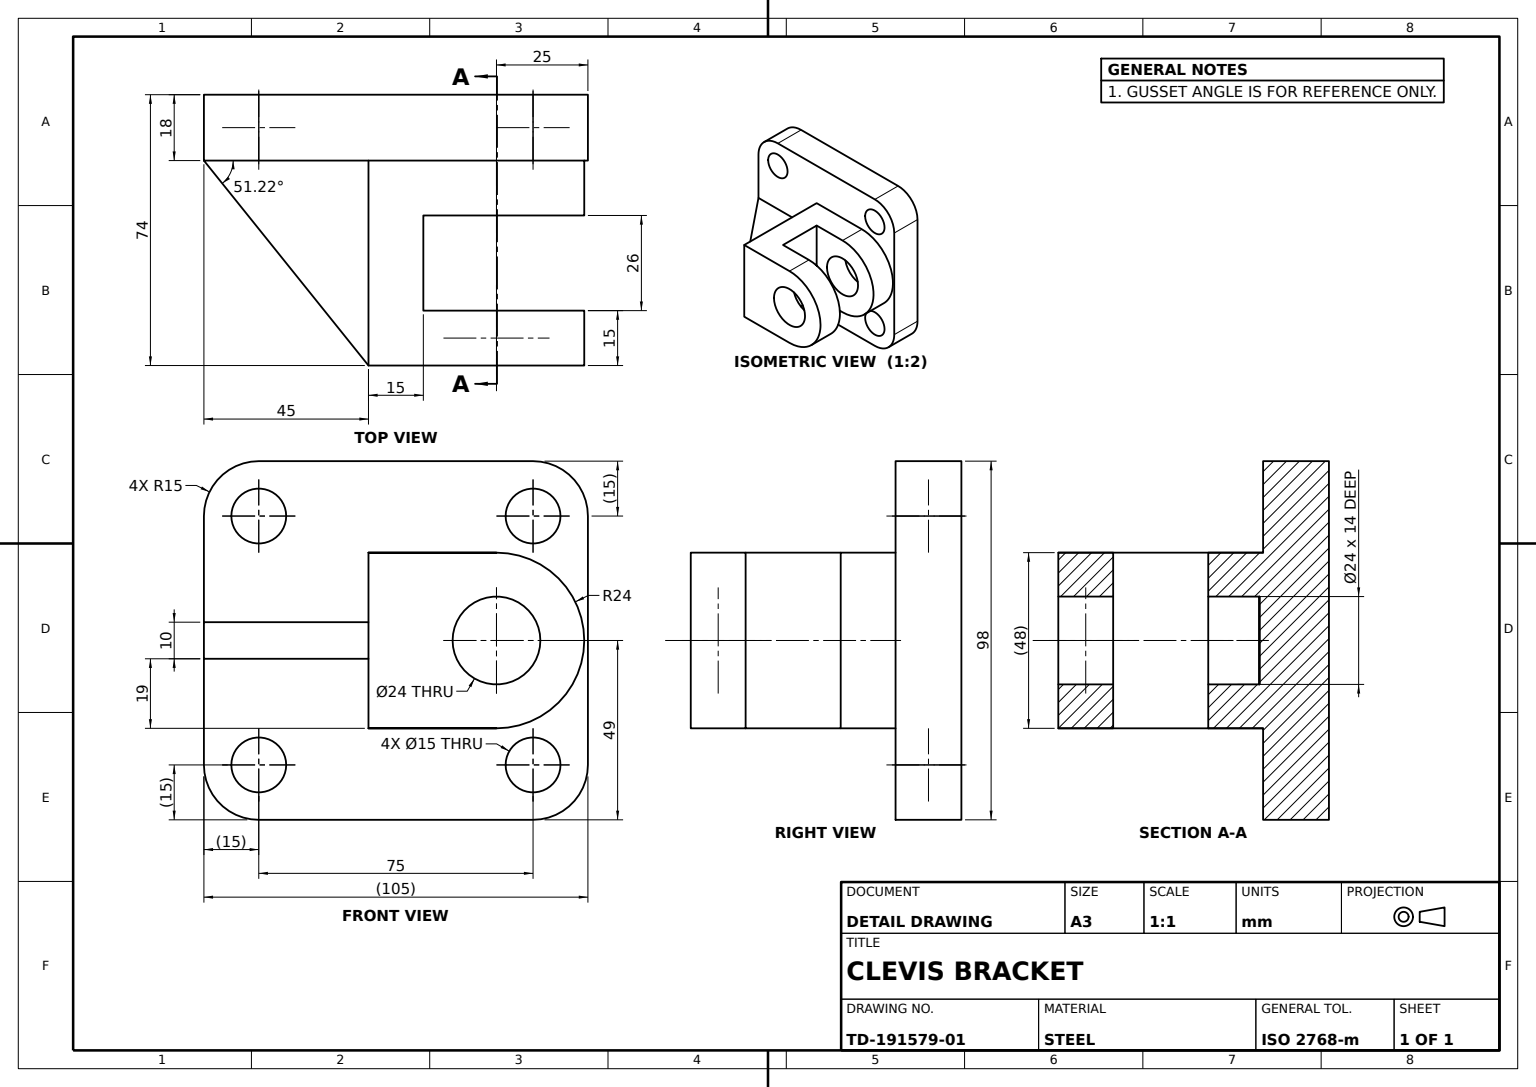
from build123d import *

# Parameters (mm, degrees)
BASE_PLATE_DEPTH           = 18
MOUNTING_HOLES_SKETCH_R    = 7.5
MOUNTING_HOLES_4X_15_DEPTH = 18
CLEVIS_BASE_BOSS_DEPTH     = 15
CLEVIS_BODY_SKETCH_W       = 10
CLEVIS_BODY_SKETCH_H       = 41
CLEVIS_BODY_DEPTH          = 48
EYE_SPACER_SKETCH_W        = 41
EYE_SPACER_SKETCH_H        = 48
EYE_SPACER_DEPTH           = 5
EYE_LUG_SKETCH_W           = 20
EYE_LUG_SKETCH_H           = 48
EYE_LUG_DEPTH              = 15
EYE_START                  = -15
EYE_LUG_ROUND_END_DEPTH    = 15
EYE_BORE_SKETCH_R          = 12
EYE_BORE_24_DEPTH          = 55
GUSSET_DEPTH               = 48
GUSSET_TRIM_A_DEPTH        = 19
GUSSET_TRIM_B_DEPTH        = 19


with BuildPart() as part:
    # Base Plate Sketch → Base Plate (new body)
    with BuildSketch(Plane.XY):
        with BuildLine():
            Line((15, 0), (90, 0))
            ThreePointArc((90, 0), (100.606601718, 4.393398282), (105, 15))
            Line((105, 15), (105, 83))
            ThreePointArc((105, 83), (100.606601718, 93.606601718), (90, 98))
            Line((90, 98), (15, 98))
            ThreePointArc((15, 98), (4.393398282, 93.606601718), (0, 83))
            Line((0, 83), (0, 15))
            ThreePointArc((0, 15), (4.393398282, 4.393398282), (15, 0))
        make_face()
    extrude(amount=BASE_PLATE_DEPTH)

    # Mounting Holes Sketch → Mounting Holes 4xØ15 (cut)
    with BuildSketch(Plane.XY.offset(18)):
        with Locations((15, 83)):
            Circle(MOUNTING_HOLES_SKETCH_R)
        with Locations((90, 83)):
            Circle(MOUNTING_HOLES_SKETCH_R)
        with Locations((90, 15)):
            Circle(MOUNTING_HOLES_SKETCH_R)
        with Locations((15, 15)):
            Circle(MOUNTING_HOLES_SKETCH_R)
    extrude(amount=-MOUNTING_HOLES_4X_15_DEPTH, mode=Mode.SUBTRACT)

    # Clevis Base Boss Sketch → Clevis Base Boss (add)
    with BuildSketch(Plane.XY.offset(18)):
        with BuildLine():
            Line((80, 73), (45, 73))
            Line((45, 73), (45, 25))
            Line((45, 25), (80, 25))
            ThreePointArc((80, 25), (104, 49), (80, 73))
        make_face()
    extrude(amount=CLEVIS_BASE_BOSS_DEPTH)

    # Clevis Body Sketch → Clevis Body (add)
    with BuildSketch(Plane.XZ.offset(-25)):
        with Locations((50, 53.5)):
            Rectangle(CLEVIS_BODY_SKETCH_W, CLEVIS_BODY_SKETCH_H)
    extrude(amount=-CLEVIS_BODY_DEPTH)

    # Eye Spacer Sketch → Eye Spacer (add)
    with BuildSketch(Plane(origin=(55, 0, 0), x_dir=(0, 0, -1), z_dir=(1, 0, 0))):
        with Locations((-53.5, 49)):
            Rectangle(EYE_SPACER_SKETCH_W, EYE_SPACER_SKETCH_H)
    extrude(amount=EYE_SPACER_DEPTH)

    # Eye Lug Sketch → Eye Lug (add)
    with BuildSketch(Plane.XY.offset(74)):
        with Locations((70, 49)):
            Rectangle(EYE_LUG_SKETCH_W, EYE_LUG_SKETCH_H)
    extrude(amount=-EYE_LUG_DEPTH)

    # Eye Lug Round End Sketch → Eye Lug Round End (add)
    with BuildSketch(Plane.XY.offset(74).offset(EYE_START)):
        with BuildLine():
            Line((80, 73), (80, 25))
            ThreePointArc((80, 25), (104, 49), (80, 73))
        make_face()
    extrude(amount=EYE_LUG_ROUND_END_DEPTH)

    # Eye Bore Sketch → Eye Bore Ø24 (cut)
    with BuildSketch(Plane.XY.offset(74)):
        with Locations((80, 49)):
            Circle(EYE_BORE_SKETCH_R)
    extrude(amount=-EYE_BORE_24_DEPTH, mode=Mode.SUBTRACT)

    # Gusset Sketch → Gusset (add)
    with BuildSketch(Plane.XZ.offset(-25)):
        Polygon((45, 74), (45, 18), (0, 18), align=None)
    extrude(amount=-GUSSET_DEPTH)

    # Gusset Trim A Sketch → Gusset Trim A (cut)
    with BuildSketch(Plane.XZ.offset(-25)):
        Polygon((45, 74), (45, 18), (0, 18), align=None)
    extrude(amount=-GUSSET_TRIM_A_DEPTH, mode=Mode.SUBTRACT)

    # Gusset Trim B Sketch → Gusset Trim B (cut)
    with BuildSketch(Plane(origin=(0, 73, 0), x_dir=(1, 0, 0), z_dir=(0, 1, 0))):
        Polygon((45, -74), (45, -18), (0, -18), align=None)
    extrude(amount=-GUSSET_TRIM_B_DEPTH, mode=Mode.SUBTRACT)


solid = part.part
